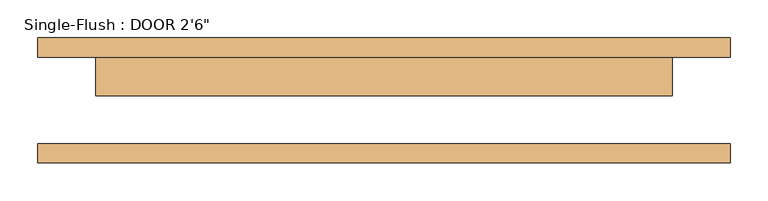
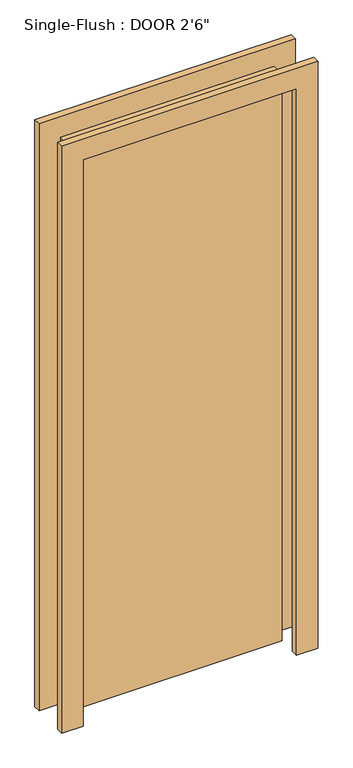
"""IFC4 building model written with IfcOpenShell, lengths in millimetres: door geometry."""

from ifc_helpers import new_model, si_unit, frame, origin, origin_with_axes, place, context, project, spatial, polyline, outline, extrude, source, transform, mapped, element, save


def door_214872d5(model_context):
    return source(origin(), model_context, "Body", "SweptSolid", [
        extrude(outline(polyline([(2209.8, -457.2), (0.0, -457.2), (0.0, -381.0), (2133.6, -381.0), (2133.6, 381.0), (0.0, 381.0), (0.0, 457.2), (2209.8, 457.2), (2209.8, -457.2)])), frame((0.0, 57.15, 0.0), z_axis=(0.0, 1.0, 0.0), x_axis=(0.0, 0.0, 1.0)), (0.0, 0.0, 1.0), 25.4),
        extrude(outline(polyline([(2209.8, 457.2), (2209.8, -457.2), (0.0, -457.2), (0.0, -381.0), (2133.6, -381.0), (2133.6, 381.0), (0.0, 381.0), (0.0, 457.2), (2209.8, 457.2)])), frame((0.0, -82.55, 0.0), z_axis=(0.0, 1.0, 0.0), x_axis=(0.0, 0.0, 1.0)), (0.0, 0.0, 1.0), 25.4),
        extrude(outline(polyline([(381.0, 6.35), (-381.0, 6.35), (-381.0, 57.15), (381.0, 57.15), (381.0, 6.35)])), origin_with_axes(), (0.0, 0.0, 1.0), 2133.6),
    ])


if __name__ == "__main__":
    model = new_model("IFC4")
    model_context = context("Model", 3, world=origin())
    ifc_project = project(units=[si_unit("LENGTHUNIT", "METRE", prefix="MILLI")], contexts=[model_context])
    site = spatial("IfcSite", under=ifc_project)
    building = spatial("IfcBuilding", under=site)
    placement = place(None, origin())
    door_shape = door_214872d5(model_context)
    element("IfcDoor", 1, ObjectType="Single-Flush : DOOR 2'6\"", at=placement, inside=building, context=model_context, shape_type="MappedRepresentation", body=[
        mapped(door_shape, transform((0.0, 0.0, 0.0), x_axis=(1.0, 0.0, 0.0), y_axis=(0.0, 1.0, 0.0), z_axis=(0.0, 0.0, 1.0))),
    ])
    save(model, "model.ifc")

# Revit data of these elements
# Type "Single-Flush : DOOR 2'6\""
#   Type Mark = "10"
#   Construction Type Id = "MDOOR"
#   Assembly Code = "C1020"
#   Analytic Construction = "Metal"
#   Thickness = 0' - 2"
#   Heat Transfer Coefficient (U) = 0.651978 BTU/(h·ft²·°F)
#   Height = 7' - 0"
#   Trim Projection Ext = 0' - 1"
#   Trim Projection Int = 0' - 1"
#   Trim Width = 0' - 3"
#   Width = 2' - 6"
#   Define Thermal Properties by = 1
#   Door Material = Door - Panel
#   Frame Material = Door - Frame
#   Visual Light Transmittance = 0
#   Solar Heat Gain Coefficient = 0
#   Function = (empty or 0)
#   Wall Closure = (empty or 0)
# Element 1 (IfcDoor, "Single-Flush : DOOR 2'6\"")
#   Materials on its faces: "Door - Frame", "Door - Panel"
# Materials
#   "Door - Panel": class "Wood", colour RGB 210 159 95, transparency 0, Cost = 0
#   "Door - Frame": colour RGB 118 70 51, transparency 0, Cost = 0
